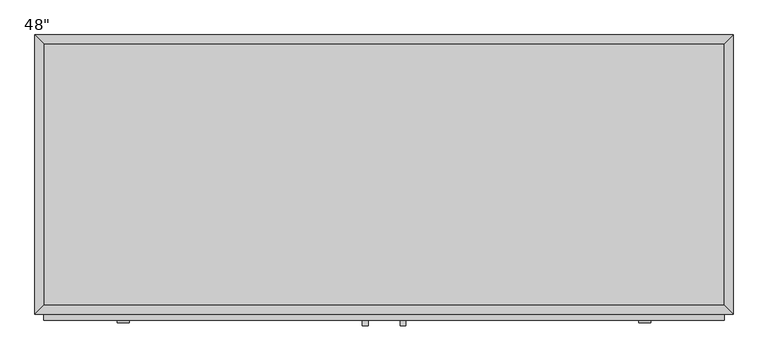
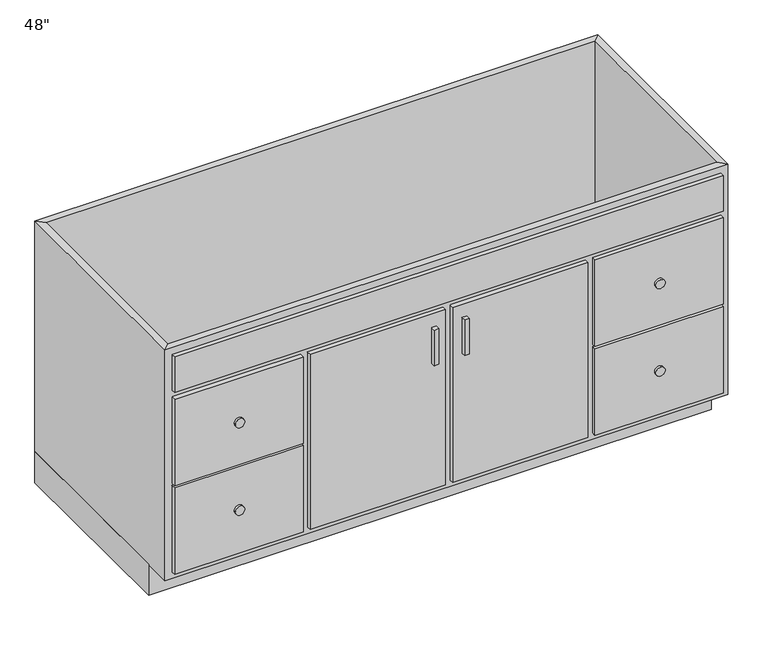
"""IFC4 building model written with IfcOpenShell, lengths in millimetres: furniture geometry."""

from ifc_helpers import new_model, si_unit, point, frame, frame_2d, origin, origin_with_axes, place, context, project, spatial, polyline, circle_curve, trimmed, segment, composite_curve, outline, extrude, faceted_brep, source, transform, mapped, element, save


def furniture_d2b2b685(model_context):
    return source(origin(), model_context, "Body", "SolidModel", [
        extrude(outline(polyline([(852.84496, 0.0), (852.84496, -533.4), (-671.15504, -533.4), (-671.15504, 0.0), (852.84496, 0.0)])), origin_with_axes(), (0.0, 0.0, 1.0), 88.9),
        faceted_brep([(833.79496, -590.55, 749.3), (833.79496, -590.55, 88.9), (-652.10504, -590.55, 88.9), (-652.10504, -590.55, 749.3), (852.84496, -609.6, 749.3), (-671.15504, -609.6, 749.3), (852.84496, -609.6, 88.9), (-671.15504, -609.6, 88.9), (-652.10504, -19.05, 88.9), (-652.10504, -19.05, 749.3), (-671.15504, 0.0, 749.3), (-671.15504, 0.0, 88.9), (833.79496, -19.05, 88.9), (833.79496, -19.05, 749.3), (852.84496, 0.0, 749.3), (852.84496, 0.0, 88.9)], [[[0, 1, 2, 3]], [[4, 0, 3, 5]], [[6, 4, 5, 7]], [[1, 6, 7, 2]], [[3, 2, 8, 9]], [[5, 3, 9, 10]], [[7, 5, 10, 11]], [[2, 7, 11, 8]], [[9, 8, 12, 13]], [[10, 9, 13, 14]], [[11, 10, 14, 15]], [[8, 11, 15, 12]], [[13, 12, 1, 0]], [[14, 13, 0, 4]], [[15, 14, 4, 6]], [[12, 15, 6, 1]]]),
        extrude(outline(polyline([(833.79496, -19.05), (833.79496, -590.55), (-652.10504, -590.55), (-652.10504, -19.05), (833.79496, -19.05)])), frame((0.0, 0.0, 88.9), z_axis=(0.0, 0.0, 1.0), x_axis=(1.0, 0.0, 0.0)), (0.0, 0.0, 1.0), 19.05),
        extrude(outline(composite_curve([segment(trimmed(circle_curve(frame_2d((233.3625, 659.96371)), 12.7), [point((233.3625, 647.26371))], [point((233.3625, 672.66371))], False, "CARTESIAN"), True, "CONTINUOUS"), segment(trimmed(circle_curve(frame_2d((233.3625, 659.96371)), 12.7), [point((233.3625, 672.66371))], [point((233.3625, 647.26371))], False, "CARTESIAN"), True, "CONTINUOUS")], self_intersect=False)), frame((0.0, -628.65, 0.0), z_axis=(0.0, 1.0, 0.0), x_axis=(0.0, 0.0, 1.0)), (0.0, 0.0, 1.0), 6.35),
        extrude(outline(composite_curve([segment(trimmed(circle_curve(frame_2d((484.1875, 659.96371)), 12.7), [point((484.1875, 647.26371))], [point((484.1875, 672.66371))], False, "CARTESIAN"), True, "CONTINUOUS"), segment(trimmed(circle_curve(frame_2d((484.1875, 659.96371)), 12.7), [point((484.1875, 672.66371))], [point((484.1875, 647.26371))], False, "CARTESIAN"), True, "CONTINUOUS")], self_intersect=False)), frame((0.0, -628.65, 0.0), z_axis=(0.0, 1.0, 0.0), x_axis=(0.0, 0.0, 1.0)), (0.0, 0.0, 1.0), 6.35),
        extrude(outline(composite_curve([segment(trimmed(circle_curve(frame_2d((484.1875, -478.27379)), 12.7), [point((484.1875, -490.97379))], [point((484.1875, -465.57379))], False, "CARTESIAN"), True, "CONTINUOUS"), segment(trimmed(circle_curve(frame_2d((484.1875, -478.27379)), 12.7), [point((484.1875, -465.57379))], [point((484.1875, -490.97379))], False, "CARTESIAN"), True, "CONTINUOUS")], self_intersect=False)), frame((0.0, -628.65, 0.0), z_axis=(0.0, 1.0, 0.0), x_axis=(0.0, 0.0, 1.0)), (0.0, 0.0, 1.0), 6.35),
        extrude(outline(composite_curve([segment(trimmed(circle_curve(frame_2d((233.3625, -478.27379)), 12.7), [point((233.3625, -490.97379))], [point((233.3625, -465.57379))], False, "CARTESIAN"), True, "CONTINUOUS"), segment(trimmed(circle_curve(frame_2d((233.3625, -478.27379)), 12.7), [point((233.3625, -465.57379))], [point((233.3625, -490.97379))], False, "CARTESIAN"), True, "CONTINUOUS")], self_intersect=False)), frame((0.0, -628.65, 0.0), z_axis=(0.0, 1.0, 0.0), x_axis=(0.0, 0.0, 1.0)), (0.0, 0.0, 1.0), 6.35),
        extrude(outline(polyline([(55.91996, -635.0), (43.21996, -635.0), (43.21996, -622.3), (55.91996, -622.3), (55.91996, -635.0)])), frame((0.0, 0.0, 469.9), z_axis=(0.0, 0.0, 1.0), x_axis=(1.0, 0.0, 0.0)), (0.0, 0.0, 1.0), 101.6),
        extrude(outline(polyline([(138.46996, -635.0), (125.76996, -635.0), (125.76996, -622.3), (138.46996, -622.3), (138.46996, -635.0)])), frame((0.0, 0.0, 469.9), z_axis=(0.0, 0.0, 1.0), x_axis=(1.0, 0.0, 0.0)), (0.0, 0.0, 1.0), 101.6),
        extrude(outline(polyline([(833.79496, -622.3), (-652.10504, -622.3), (-652.10504, -609.6), (833.79496, -609.6), (833.79496, -622.3)])), frame((0.0, 0.0, 628.65), z_axis=(0.0, 0.0, 1.0), x_axis=(1.0, 0.0, 0.0)), (0.0, 0.0, 1.0), 101.6),
        extrude(outline(polyline([(833.79496, -622.3), (486.13246, -622.3), (486.13246, -609.6), (833.79496, -609.6), (833.79496, -622.3)])), frame((0.0, 0.0, 361.95), z_axis=(0.0, 0.0, 1.0), x_axis=(1.0, 0.0, 0.0)), (0.0, 0.0, 1.0), 247.65),
        extrude(outline(polyline([(833.79496, -622.3), (486.13246, -622.3), (486.13246, -609.6), (833.79496, -609.6), (833.79496, -622.3)])), frame((0.0, 0.0, 107.95), z_axis=(0.0, 0.0, 1.0), x_axis=(1.0, 0.0, 0.0)), (0.0, 0.0, 1.0), 247.65),
        extrude(outline(polyline([(-304.44254, -622.3), (-652.10504, -622.3), (-652.10504, -609.6), (-304.44254, -609.6), (-304.44254, -622.3)])), frame((0.0, 0.0, 361.95), z_axis=(0.0, 0.0, 1.0), x_axis=(1.0, 0.0, 0.0)), (0.0, 0.0, 1.0), 247.65),
        extrude(outline(polyline([(-304.44254, -622.3), (-652.10504, -622.3), (-652.10504, -609.6), (-304.44254, -609.6), (-304.44254, -622.3)])), frame((0.0, 0.0, 107.95), z_axis=(0.0, 0.0, 1.0), x_axis=(1.0, 0.0, 0.0)), (0.0, 0.0, 1.0), 247.65),
        extrude(outline(polyline([(81.31996, -622.3), (-285.39254, -622.3), (-285.39254, -609.6), (81.31996, -609.6), (81.31996, -622.3)])), frame((0.0, 0.0, 107.95), z_axis=(0.0, 0.0, 1.0), x_axis=(1.0, 0.0, 0.0)), (0.0, 0.0, 1.0), 501.65),
        extrude(outline(polyline([(467.08246, -622.3), (100.36996, -622.3), (100.36996, -609.6), (467.08246, -609.6), (467.08246, -622.3)])), frame((0.0, 0.0, 107.95), z_axis=(0.0, 0.0, 1.0), x_axis=(1.0, 0.0, 0.0)), (0.0, 0.0, 1.0), 501.65),
    ])


if __name__ == "__main__":
    model = new_model("IFC4")
    model_context = context("Model", 3, world=origin())
    ifc_project = project(units=[si_unit("LENGTHUNIT", "METRE", prefix="MILLI")], contexts=[model_context])
    site = spatial("IfcSite", under=ifc_project)
    building = spatial("IfcBuilding", under=site)
    placement = place(None, origin())
    furniture_shape = furniture_d2b2b685(model_context)
    element("IfcFurniture", 1, ObjectType="48\"", at=placement, inside=building, context=model_context, shape_type="MappedRepresentation", body=[
        mapped(furniture_shape, transform((0.0, 0.0, 0.0), x_axis=(1.0, 0.0, 0.0), y_axis=(0.0, 1.0, 0.0), z_axis=(0.0, 0.0, 1.0))),
    ])
    save(model, "model.ifc")

# Revit data of these elements
# Type "48\""
#   Assembly Code = "C1030410"
#   Depth = 2' - 0"
#   Height = 2' - 5 1/2"
#   Toe Depth = 0' - 3"
#   Toe Height = 0' - 3 1/2"
#   Width = 5' - 0"
#   Cabinet Material = none
#   Door/Drawer Material = none
#   Handle Material = Cabinets - Handles
#   Default Elevation = 0
# Element 1 (IfcFurniture, "48\"")
#   Materials on its faces: "Cabinets - Handles", "Cabinets"
# Materials
#   "Cabinets - Handles": class "Metal", colour RGB 57 57 57, transparency 0
#   "Cabinets": colour RGB 249 249 249, transparency 0
